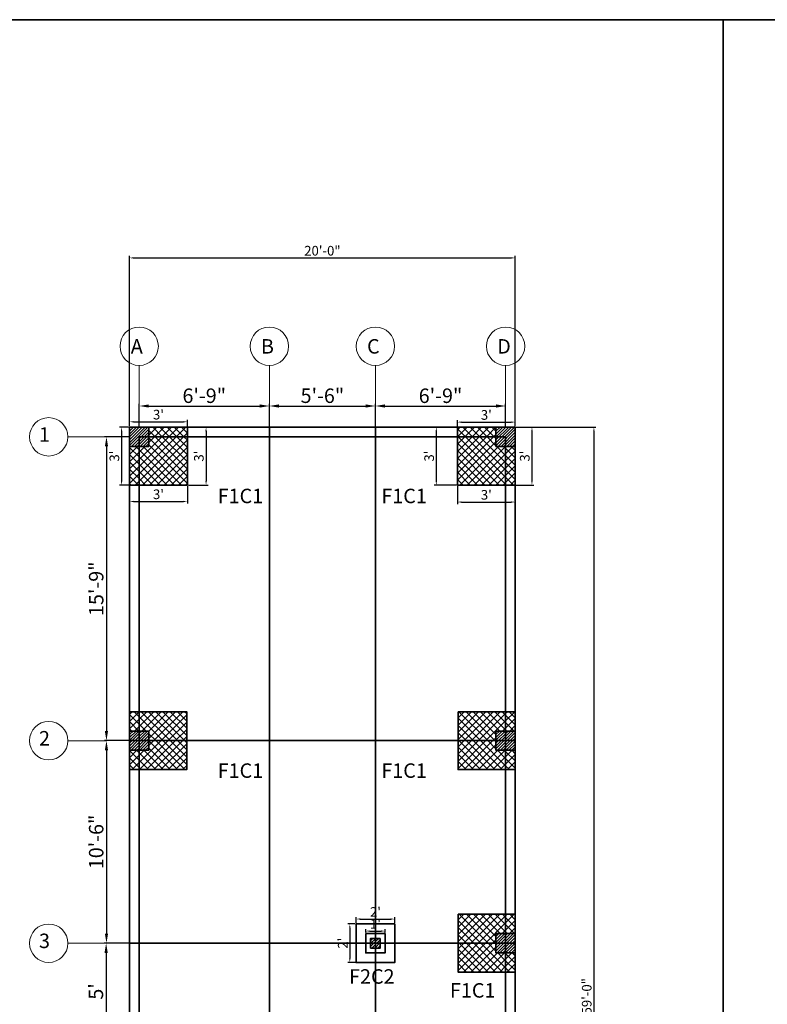
# Model space of a CAD drawing. Units: millimetres. Extents: x 20768 to 23556, y 50760 to 52704.
# Tile 35 of 36: x 22556 to 23021, y 52092 to 52704. Entities that reach past the tile are written whole.
import ezdxf

# ---------------------------------------------------------------- set-up
doc = ezdxf.new("R2010")
doc.units = ezdxf.units.MM
for name, color, linetype, lineweight in [('A-ANNO-TTLB', 7, 'Continuous', 35), ('S-ANNO-DIMS', 2, 'Continuous', 18), ('S-ANNO-TEXT', 6, 'Continuous', 18), ('S-BEAM', 3, 'Continuous', 35), ('S-COLS', 20, 'Continuous', 35), ('S-COLS-PATT', 8, 'Continuous', 13), ('S-FNDN', 200, 'Continuous', 35), ('S-GRID', 1, 'Continuous', 18)]:
    doc.layers.add(name, color=color, linetype=linetype, lineweight=lineweight)
doc.styles.get("Standard").update_dxf_attribs({"font": 'arial.ttf'})
doc.dimstyles.new('ISO-25', dxfattribs={"dimtxt": 6, "dimasz": 2.5, "dimexe": 1.25, "dimexo": 0.625, "dimtad": 1, "dimdec": 0, "dimlunit": 3, "dimtxsty": 'Standard', "dimcen": 2.5, "dimadec": 0, "dimazin": 0, "dimtfac": 1, "dimtdec": 0, "dimtmove": 0, "dimatfit": 3, "dimfxl": 1, "dimarcsym": 0})
pattern_1 = [(45, (568.6884, 0), (-0.898025612, 0.898025612), [])]
pattern_2 = [(45, (-102.8262, 0), (-2.24506403, 2.24506403), []), (135, (-102.8262, 0), (-2.24506403, -2.24506403), [])]
pattern_3 = [(45, (-102.8262, 0), (-0.898025612, 0.898025612), [])]

# ---------------------------------------------------------------- blocks, each defined once
blk = doc.blocks.new('*D51')
at = {"layer": 'Defpoints', "color": 0, "transparency": 16777216}
for p in [(22710.96, 52463.68), (22629.96, 52450.51), (22710.96, 52450.51)]:
    blk.add_point(p, dxfattribs=at)
at = {"layer": 'S-ANNO-DIMS', "color": 0, "lineweight": -2, "transparency": 16777216}
for p, q in [((22629.96, 52451.13), (22629.96, 52464.93)), ((22710.96, 52451.13), (22710.96, 52464.93)), ((22635.96, 52463.68), (22704.96, 52463.68))]:
    blk.add_line(p, q, dxfattribs=at)
at = {"layer": 'S-ANNO-DIMS', "color": 0, "transparency": 16777216}
for points in [[(22635.96, 52464.68), (22635.96, 52462.68), (22629.96, 52463.68)], [(22704.96, 52464.68), (22704.96, 52462.68), (22710.96, 52463.68)]]:
    blk.add_solid(points, dxfattribs=at)
at = {"layer": 'S-ANNO-DIMS', "color": 0, "transparency": 16777216, "insert": (22670.46, 52468.9), "char_height": 9, "attachment_point": 5}
blk.add_mtext('6\'-9"', dxfattribs=at)
blk = doc.blocks.new('*D52')
at = {"layer": 'Defpoints', "color": 0, "transparency": 16777216}
for p in [(22776.96, 52463.68), (22710.96, 52450.51), (22776.96, 52450.51)]:
    blk.add_point(p, dxfattribs=at)
at = {"layer": 'S-ANNO-DIMS', "color": 0, "lineweight": -2, "transparency": 16777216}
for p, q in [((22710.96, 52451.13), (22710.96, 52464.93)), ((22776.96, 52451.13), (22776.96, 52464.93)), ((22716.96, 52463.68), (22770.96, 52463.68))]:
    blk.add_line(p, q, dxfattribs=at)
at = {"layer": 'S-ANNO-DIMS', "color": 0, "transparency": 16777216}
for points in [[(22716.96, 52464.68), (22716.96, 52462.68), (22710.96, 52463.68)], [(22770.96, 52464.68), (22770.96, 52462.68), (22776.96, 52463.68)]]:
    blk.add_solid(points, dxfattribs=at)
at = {"layer": 'S-ANNO-DIMS', "color": 0, "transparency": 16777216, "insert": (22743.96, 52468.9), "char_height": 9, "attachment_point": 5}
blk.add_mtext('5\'-6"', dxfattribs=at)
blk = doc.blocks.new('*D53')
at = {"layer": 'Defpoints', "color": 0, "transparency": 16777216}
for p in [(22857.96, 52463.68), (22776.96, 52450.51), (22857.96, 52450.51)]:
    blk.add_point(p, dxfattribs=at)
at = {"layer": 'S-ANNO-DIMS', "color": 0, "lineweight": -2, "transparency": 16777216}
for p, q in [((22776.96, 52451.13), (22776.96, 52464.93)), ((22857.96, 52451.13), (22857.96, 52464.93)), ((22782.96, 52463.68), (22851.96, 52463.68))]:
    blk.add_line(p, q, dxfattribs=at)
at = {"layer": 'S-ANNO-DIMS', "color": 0, "transparency": 16777216}
for points in [[(22782.96, 52464.68), (22782.96, 52462.68), (22776.96, 52463.68)], [(22851.96, 52464.68), (22851.96, 52462.68), (22857.96, 52463.68)]]:
    blk.add_solid(points, dxfattribs=at)
at = {"layer": 'S-ANNO-DIMS', "color": 0, "transparency": 16777216, "insert": (22817.46, 52468.9), "char_height": 9, "attachment_point": 5}
blk.add_mtext('6\'-9"', dxfattribs=at)
blk = doc.blocks.new('*D54')
at = {"layer": 'Defpoints', "color": 0, "transparency": 16777216}
for p in [(22623.96, 52444.51), (22609.6, 52255.51), (22623.96, 52255.51)]:
    blk.add_point(p, dxfattribs=at)
at = {"layer": 'S-ANNO-DIMS', "color": 0, "lineweight": -2, "transparency": 16777216}
for p, q in [((22623.34, 52444.51), (22608.35, 52444.51)), ((22609.6, 52438.51), (22609.6, 52261.51)), ((22623.34, 52255.51), (22608.35, 52255.51))]:
    blk.add_line(p, q, dxfattribs=at)
at = {"layer": 'S-ANNO-DIMS', "color": 0, "transparency": 16777216}
for points in [[(22608.6, 52438.51), (22610.6, 52438.51), (22609.6, 52444.51)], [(22608.6, 52261.51), (22610.6, 52261.51), (22609.6, 52255.51)]]:
    blk.add_solid(points, dxfattribs=at)
at = {"layer": 'S-ANNO-DIMS', "color": 0, "transparency": 16777216, "insert": (22604.38, 52350.01), "char_height": 9, "attachment_point": 5, "rotation": 90}
blk.add_mtext('15\'-9"', dxfattribs=at)
blk = doc.blocks.new('*D55')
at = {"layer": 'Defpoints', "color": 0, "transparency": 16777216}
for p in [(22623.96, 52255.51), (22609.6, 52129.51), (22623.96, 52129.51)]:
    blk.add_point(p, dxfattribs=at)
at = {"layer": 'S-ANNO-DIMS', "color": 0, "lineweight": -2, "transparency": 16777216}
for p, q in [((22623.34, 52255.51), (22608.35, 52255.51)), ((22609.6, 52249.51), (22609.6, 52135.51)), ((22623.34, 52129.51), (22608.35, 52129.51))]:
    blk.add_line(p, q, dxfattribs=at)
at = {"layer": 'S-ANNO-DIMS', "color": 0, "transparency": 16777216}
for points in [[(22608.6, 52249.51), (22610.6, 52249.51), (22609.6, 52255.51)], [(22608.6, 52135.51), (22610.6, 52135.51), (22609.6, 52129.51)]]:
    blk.add_solid(points, dxfattribs=at)
at = {"layer": 'S-ANNO-DIMS', "color": 0, "transparency": 16777216, "insert": (22604.38, 52192.51), "char_height": 9, "attachment_point": 5, "rotation": 90}
blk.add_mtext('10\'-6"', dxfattribs=at)
blk = doc.blocks.new('*D56')
at = {"layer": 'Defpoints', "color": 0, "transparency": 16777216}
for p in [(22623.96, 52129.51), (22609.39, 52069.51), (22623.96, 52069.51)]:
    blk.add_point(p, dxfattribs=at)
at = {"layer": 'S-ANNO-DIMS', "color": 0, "lineweight": -2, "transparency": 16777216}
for p, q in [((22623.34, 52129.51), (22608.14, 52129.51)), ((22609.39, 52123.51), (22609.39, 52075.51)), ((22623.34, 52069.51), (22608.14, 52069.51))]:
    blk.add_line(p, q, dxfattribs=at)
at = {"layer": 'S-ANNO-DIMS', "color": 0, "transparency": 16777216}
for points in [[(22608.39, 52123.51), (22610.39, 52123.51), (22609.39, 52129.51)], [(22608.39, 52075.51), (22610.39, 52075.51), (22609.39, 52069.51)]]:
    blk.add_solid(points, dxfattribs=at)
at = {"layer": 'S-ANNO-DIMS', "color": 0, "transparency": 16777216, "insert": (22604.19, 52099.51), "char_height": 9, "attachment_point": 5, "rotation": 90}
blk.add_mtext("5'", dxfattribs=at)
blk = doc.blocks.new('*D59')
at = {"layer": 'Defpoints', "color": 0, "transparency": 16777216}
for p in [(22623.96, 52414.51), (22659.96, 52414.51), (22659.96, 52404.3)]:
    blk.add_point(p, dxfattribs=at)
at = {"layer": 'S-ANNO-DIMS', "color": 0, "lineweight": -2, "transparency": 16777216}
for p, q in [((22623.96, 52413.88), (22623.96, 52403.05)), ((22659.96, 52413.88), (22659.96, 52403.05)), ((22626.46, 52404.3), (22657.46, 52404.3))]:
    blk.add_line(p, q, dxfattribs=at)
at = {"layer": 'S-ANNO-DIMS', "color": 0, "transparency": 16777216}
for points in [[(22626.46, 52404.72), (22626.46, 52403.89), (22623.96, 52404.3)], [(22657.46, 52404.72), (22657.46, 52403.89), (22659.96, 52404.3)]]:
    blk.add_solid(points, dxfattribs=at)
at = {"layer": 'S-ANNO-DIMS', "color": 0, "transparency": 16777216, "insert": (22641.96, 52407.99), "char_height": 6, "attachment_point": 5}
blk.add_mtext("3'", dxfattribs=at)
blk = doc.blocks.new('*D60')
at = {"layer": 'Defpoints', "color": 0, "transparency": 16777216}
for p in [(22659.96, 52450.51), (22659.96, 52414.51), (22671.57, 52414.51)]:
    blk.add_point(p, dxfattribs=at)
at = {"layer": 'S-ANNO-DIMS', "color": 0, "lineweight": -2, "transparency": 16777216}
for p, q in [((22660.59, 52450.51), (22672.82, 52450.51)), ((22671.57, 52448.01), (22671.57, 52417.01)), ((22660.59, 52414.51), (22672.82, 52414.51))]:
    blk.add_line(p, q, dxfattribs=at)
at = {"layer": 'S-ANNO-DIMS', "color": 0, "transparency": 16777216}
for points in [[(22671.15, 52448.01), (22671.98, 52448.01), (22671.57, 52450.51)], [(22671.15, 52417.01), (22671.98, 52417.01), (22671.57, 52414.51)]]:
    blk.add_solid(points, dxfattribs=at)
at = {"layer": 'S-ANNO-DIMS', "color": 0, "transparency": 16777216, "insert": (22667.88, 52432.51), "char_height": 6, "attachment_point": 5, "rotation": 90}
blk.add_mtext("3'", dxfattribs=at)
blk = doc.blocks.new('*D61')
at = {"layer": 'Defpoints', "color": 0, "transparency": 16777216}
for p in [(22659.96, 52453.85), (22623.96, 52450.51), (22659.96, 52450.51)]:
    blk.add_point(p, dxfattribs=at)
at = {"layer": 'S-ANNO-DIMS', "color": 0, "lineweight": -2, "transparency": 16777216}
for p, q in [((22623.96, 52451.13), (22623.96, 52455.1)), ((22626.46, 52453.85), (22657.46, 52453.85)), ((22659.96, 52451.13), (22659.96, 52455.1))]:
    blk.add_line(p, q, dxfattribs=at)
at = {"layer": 'S-ANNO-DIMS', "color": 0, "transparency": 16777216}
for points in [[(22626.46, 52454.27), (22626.46, 52453.43), (22623.96, 52453.85)], [(22657.46, 52454.27), (22657.46, 52453.43), (22659.96, 52453.85)]]:
    blk.add_solid(points, dxfattribs=at)
at = {"layer": 'S-ANNO-DIMS', "color": 0, "transparency": 16777216, "insert": (22641.96, 52457.54), "char_height": 6, "attachment_point": 5}
blk.add_mtext("3'", dxfattribs=at)
blk = doc.blocks.new('*D48')
at = {"layer": 'Defpoints', "color": 0, "transparency": 16777216}
for p in [(22623.96, 52450.51), (22619.01, 52414.51), (22623.96, 52414.51)]:
    blk.add_point(p, dxfattribs=at)
at = {"layer": 'S-ANNO-DIMS', "color": 0, "lineweight": -2, "transparency": 16777216}
for p, q in [((22623.34, 52450.51), (22617.76, 52450.51)), ((22619.01, 52448.01), (22619.01, 52417.01)), ((22623.34, 52414.51), (22617.76, 52414.51))]:
    blk.add_line(p, q, dxfattribs=at)
at = {"layer": 'S-ANNO-DIMS', "color": 0, "transparency": 16777216}
for points in [[(22618.59, 52448.01), (22619.42, 52448.01), (22619.01, 52450.51)], [(22618.59, 52417.01), (22619.42, 52417.01), (22619.01, 52414.51)]]:
    blk.add_solid(points, dxfattribs=at)
at = {"layer": 'S-ANNO-DIMS', "color": 0, "transparency": 16777216, "insert": (22615.31, 52432.51), "char_height": 6, "attachment_point": 5, "rotation": 90}
blk.add_mtext("3'", dxfattribs=at)
blk = doc.blocks.new('*D62')
at = {"layer": 'Defpoints', "color": 0, "transparency": 16777216}
for p in [(22827.96, 52450.51), (22814.83, 52414.51), (22827.96, 52414.51)]:
    blk.add_point(p, dxfattribs=at)
at = {"layer": 'S-ANNO-DIMS', "color": 0, "lineweight": -2, "transparency": 16777216}
for p, q in [((22827.34, 52450.51), (22813.58, 52450.51)), ((22814.83, 52448.01), (22814.83, 52417.01)), ((22827.34, 52414.51), (22813.58, 52414.51))]:
    blk.add_line(p, q, dxfattribs=at)
at = {"layer": 'S-ANNO-DIMS', "color": 0, "transparency": 16777216}
for points in [[(22814.41, 52448.01), (22815.25, 52448.01), (22814.83, 52450.51)], [(22814.41, 52417.01), (22815.25, 52417.01), (22814.83, 52414.51)]]:
    blk.add_solid(points, dxfattribs=at)
at = {"layer": 'S-ANNO-DIMS', "color": 0, "transparency": 16777216, "insert": (22811.14, 52432.51), "char_height": 6, "attachment_point": 5, "rotation": 90}
blk.add_mtext("3'", dxfattribs=at)
blk = doc.blocks.new('*D63')
at = {"layer": 'Defpoints', "color": 0, "transparency": 16777216}
for p in [(22827.96, 52414.51), (22863.96, 52414.51), (22863.96, 52403.95)]:
    blk.add_point(p, dxfattribs=at)
at = {"layer": 'S-ANNO-DIMS', "color": 0, "lineweight": -2, "transparency": 16777216}
for p, q in [((22827.96, 52413.88), (22827.96, 52402.7)), ((22863.96, 52413.88), (22863.96, 52402.7)), ((22830.46, 52403.95), (22861.46, 52403.95))]:
    blk.add_line(p, q, dxfattribs=at)
at = {"layer": 'S-ANNO-DIMS', "color": 0, "transparency": 16777216}
for points in [[(22830.46, 52404.37), (22830.46, 52403.54), (22827.96, 52403.95)], [(22861.46, 52404.37), (22861.46, 52403.54), (22863.96, 52403.95)]]:
    blk.add_solid(points, dxfattribs=at)
at = {"layer": 'S-ANNO-DIMS', "color": 0, "transparency": 16777216, "insert": (22845.96, 52407.64), "char_height": 6, "attachment_point": 5}
blk.add_mtext("3'", dxfattribs=at)
blk = doc.blocks.new('*D64')
at = {"layer": 'Defpoints', "color": 0, "transparency": 16777216}
for p in [(22863.96, 52450.51), (22863.96, 52414.51), (22874.35, 52414.51)]:
    blk.add_point(p, dxfattribs=at)
at = {"layer": 'S-ANNO-DIMS', "color": 0, "lineweight": -2, "transparency": 16777216}
for p, q in [((22864.59, 52450.51), (22875.6, 52450.51)), ((22874.35, 52448.01), (22874.35, 52417.01)), ((22864.59, 52414.51), (22875.6, 52414.51))]:
    blk.add_line(p, q, dxfattribs=at)
at = {"layer": 'S-ANNO-DIMS', "color": 0, "transparency": 16777216}
for points in [[(22873.93, 52448.01), (22874.77, 52448.01), (22874.35, 52450.51)], [(22873.93, 52417.01), (22874.77, 52417.01), (22874.35, 52414.51)]]:
    blk.add_solid(points, dxfattribs=at)
at = {"layer": 'S-ANNO-DIMS', "color": 0, "transparency": 16777216, "insert": (22870.66, 52432.51), "char_height": 6, "attachment_point": 5, "rotation": 90}
blk.add_mtext("3'", dxfattribs=at)
blk = doc.blocks.new('*D49')
at = {"layer": 'Defpoints', "color": 0, "transparency": 16777216}
for p in [(22863.96, 52453.66), (22827.96, 52450.51), (22863.96, 52450.51)]:
    blk.add_point(p, dxfattribs=at)
at = {"layer": 'S-ANNO-DIMS', "color": 0, "lineweight": -2, "transparency": 16777216}
for p, q in [((22827.96, 52451.13), (22827.96, 52454.91)), ((22830.46, 52453.66), (22861.46, 52453.66)), ((22863.96, 52451.13), (22863.96, 52454.91))]:
    blk.add_line(p, q, dxfattribs=at)
at = {"layer": 'S-ANNO-DIMS', "color": 0, "transparency": 16777216}
for points in [[(22830.46, 52454.08), (22830.46, 52453.24), (22827.96, 52453.66)], [(22861.46, 52454.08), (22861.46, 52453.24), (22863.96, 52453.66)]]:
    blk.add_solid(points, dxfattribs=at)
at = {"layer": 'S-ANNO-DIMS', "color": 0, "transparency": 16777216, "insert": (22845.96, 52457.35), "char_height": 6, "attachment_point": 5}
blk.add_mtext("3'", dxfattribs=at)
blk = doc.blocks.new('*D65')
at = {"layer": 'Defpoints', "color": 0, "transparency": 16777216}
for p in [(22770.96, 52135.51), (22782.96, 52137.07), (22782.96, 52135.51)]:
    blk.add_point(p, dxfattribs=at)
at = {"layer": 'S-ANNO-DIMS', "color": 0, "lineweight": -2, "transparency": 16777216}
for p, q in [((22770.96, 52136.13), (22770.96, 52138.32)), ((22773.46, 52137.07), (22780.46, 52137.07)), ((22782.96, 52136.13), (22782.96, 52138.32))]:
    blk.add_line(p, q, dxfattribs=at)
at = {"layer": 'S-ANNO-DIMS', "color": 0, "transparency": 16777216}
for points in [[(22773.46, 52137.48), (22773.46, 52136.65), (22770.96, 52137.07)], [(22780.46, 52137.48), (22780.46, 52136.65), (22782.96, 52137.07)]]:
    blk.add_solid(points, dxfattribs=at)
at = {"layer": 'S-ANNO-DIMS', "color": 0, "transparency": 16777216, "insert": (22776.96, 52140.7), "char_height": 6, "attachment_point": 5}
blk.add_mtext("1'", dxfattribs=at)
blk = doc.blocks.new('*D66')
at = {"layer": 'Defpoints', "color": 0, "transparency": 16777216}
for p in [(22764.96, 52141.51), (22788.96, 52144.54), (22788.96, 52141.51)]:
    blk.add_point(p, dxfattribs=at)
at = {"layer": 'S-ANNO-DIMS', "color": 0, "lineweight": -2, "transparency": 16777216}
for p, q in [((22764.96, 52142.13), (22764.96, 52145.79)), ((22767.46, 52144.54), (22786.46, 52144.54)), ((22788.96, 52142.13), (22788.96, 52145.79))]:
    blk.add_line(p, q, dxfattribs=at)
at = {"layer": 'S-ANNO-DIMS', "color": 0, "transparency": 16777216}
for points in [[(22767.46, 52144.95), (22767.46, 52144.12), (22764.96, 52144.54)], [(22786.46, 52144.95), (22786.46, 52144.12), (22788.96, 52144.54)]]:
    blk.add_solid(points, dxfattribs=at)
at = {"layer": 'S-ANNO-DIMS', "color": 0, "transparency": 16777216, "insert": (22776.96, 52148.17), "char_height": 6, "attachment_point": 5}
blk.add_mtext("2'", dxfattribs=at)
blk = doc.blocks.new('*D67')
at = {"layer": 'Defpoints', "color": 0, "transparency": 16777216}
for p in [(22764.96, 52141.51), (22761.03, 52117.51), (22764.96, 52117.51)]:
    blk.add_point(p, dxfattribs=at)
at = {"layer": 'S-ANNO-DIMS', "color": 0, "lineweight": -2, "transparency": 16777216}
for p, q in [((22764.34, 52141.51), (22759.78, 52141.51)), ((22761.03, 52139.01), (22761.03, 52120.01)), ((22764.34, 52117.51), (22759.78, 52117.51))]:
    blk.add_line(p, q, dxfattribs=at)
at = {"layer": 'S-ANNO-DIMS', "color": 0, "transparency": 16777216}
for points in [[(22760.61, 52139.01), (22761.44, 52139.01), (22761.03, 52141.51)], [(22760.61, 52120.01), (22761.44, 52120.01), (22761.03, 52117.51)]]:
    blk.add_solid(points, dxfattribs=at)
at = {"layer": 'S-ANNO-DIMS', "color": 0, "transparency": 16777216, "insert": (22757.39, 52129.51), "char_height": 6, "attachment_point": 5, "rotation": 90}
blk.add_mtext("2'", dxfattribs=at)
blk = doc.blocks.new('GRID-BUBBLE')
blk.add_line((47.87, 11.93), (23.87, 11.93))
blk.add_circle((11.93, 11.93), 11.93)
blk = doc.blocks.new('*D225')
at = {"layer": 'Defpoints', "color": 0, "transparency": 16777216}
for p in [(22863.96, 52555.8), (22623.96, 52450.51), (22863.96, 52450.51)]:
    blk.add_point(p, dxfattribs=at)
at = {"layer": 'S-ANNO-DIMS', "color": 0, "lineweight": -2, "transparency": 16777216}
for p, q in [((22623.96, 52451.13), (22623.96, 52557.05)), ((22863.96, 52451.13), (22863.96, 52557.05)), ((22626.46, 52555.8), (22861.46, 52555.8))]:
    blk.add_line(p, q, dxfattribs=at)
at = {"layer": 'S-ANNO-DIMS', "color": 0, "transparency": 16777216}
for points in [[(22626.46, 52556.22), (22626.46, 52555.38), (22623.96, 52555.8)], [(22861.46, 52556.22), (22861.46, 52555.38), (22863.96, 52555.8)]]:
    blk.add_solid(points, dxfattribs=at)
at = {"layer": 'S-ANNO-DIMS', "color": 0, "transparency": 16777216, "insert": (22743.96, 52559.49), "char_height": 6, "attachment_point": 5}
blk.add_mtext('20\'-0"', dxfattribs=at)
blk = doc.blocks.new('*D226')
at = {"layer": 'Defpoints', "color": 0, "transparency": 16777216}
for p in [(22863.96, 52450.51), (22863.96, 51742.51), (22912.89, 51742.51)]:
    blk.add_point(p, dxfattribs=at)
at = {"layer": 'S-ANNO-DIMS', "color": 0, "lineweight": -2, "transparency": 16777216}
for p, q in [((22864.59, 52450.51), (22914.14, 52450.51)), ((22912.89, 52448.01), (22912.89, 51745.01)), ((22864.59, 51742.51), (22914.14, 51742.51))]:
    blk.add_line(p, q, dxfattribs=at)
at = {"layer": 'S-ANNO-DIMS', "color": 0, "transparency": 16777216}
for points in [[(22912.48, 52448.01), (22913.31, 52448.01), (22912.89, 52450.51)], [(22912.48, 51745.01), (22913.31, 51745.01), (22912.89, 51742.51)]]:
    blk.add_solid(points, dxfattribs=at)
at = {"layer": 'S-ANNO-DIMS', "color": 0, "transparency": 16777216, "insert": (22909.21, 52096.51), "char_height": 6, "attachment_point": 5, "rotation": 90}
blk.add_mtext('59\'-0"', dxfattribs=at)

msp = doc.modelspace()

# ---------------------------------------------------------------- hatches: boundary and pattern name
at = {"layer": 'S-COLS-PATT'}
h = msp.add_hatch(dxfattribs=at)
h.set_pattern_fill('ANSI31', color=256, scale=0.4)
h.set_pattern_definition(pattern_1)
h.paths.add_polyline_path([(22635.96, 52450.51), (22623.96, 52450.51), (22623.96, 52438.51), (22629.96, 52438.51), (22629.96, 52444.51), (22635.96, 52444.51)])
h = msp.add_hatch(dxfattribs=at)
h.set_pattern_fill('ANSI37', color=256)
h.set_pattern_definition(pattern_2)
h.paths.add_polyline_path([(22659.96, 52450.51), (22635.96, 52450.51), (22635.96, 52444.51), (22659.96, 52444.51)])
h = msp.add_hatch(dxfattribs=at)
h.set_pattern_fill('ANSI37', color=256)
h.set_pattern_definition(pattern_2)
h.paths.add_polyline_path([(22851.96, 52450.51), (22827.96, 52450.51), (22827.96, 52444.51), (22851.96, 52444.51)])
h = msp.add_hatch(dxfattribs=at)
h.set_pattern_fill('ANSI31', color=256, scale=0.4)
h.set_pattern_definition(pattern_1)
h.paths.add_polyline_path([(22863.96, 52450.51), (22851.96, 52450.51), (22851.96, 52438.51), (22863.96, 52438.51)])
h = msp.add_hatch(dxfattribs=at)
h.set_pattern_fill('ANSI31', color=256, scale=0.4)
h.set_pattern_definition(pattern_1)
h.paths.add_polyline_path([(22635.96, 52444.51), (22629.96, 52444.51), (22629.96, 52438.51), (22635.96, 52438.51)], flags=17)
h = msp.add_hatch(dxfattribs=at)
h.set_pattern_fill('ANSI37', color=256)
h.set_pattern_definition(pattern_2)
h.paths.add_polyline_path([(22659.96, 52444.51), (22635.96, 52444.51), (22635.96, 52438.51), (22629.96, 52438.51), (22629.96, 52414.51), (22659.96, 52414.51)])
h = msp.add_hatch(dxfattribs=at)
h.set_pattern_fill('ANSI37', color=256)
h.set_pattern_definition(pattern_2)
h.paths.add_polyline_path([(22857.96, 52438.51), (22851.96, 52438.51), (22851.96, 52444.51), (22827.96, 52444.51), (22827.96, 52414.51), (22857.96, 52414.51)])
h = msp.add_hatch(dxfattribs=at)
h.set_pattern_fill('ANSI37', color=256)
h.set_pattern_definition(pattern_2)
h.paths.add_polyline_path([(22629.96, 52438.51), (22623.96, 52438.51), (22623.96, 52414.51), (22629.96, 52414.51)])
h = msp.add_hatch(dxfattribs=at)
h.set_pattern_fill('ANSI37', color=256)
h.set_pattern_definition(pattern_2)
h.paths.add_polyline_path([(22863.96, 52438.51), (22857.96, 52438.51), (22857.96, 52414.51), (22863.96, 52414.51)])
h = msp.add_hatch(dxfattribs=at)
h.set_pattern_fill('ANSI37', color=256)
h.set_pattern_definition(pattern_2)
h.paths.add_polyline_path([(22629.96, 52273.51), (22623.96, 52273.51), (22623.96, 52261.51), (22629.96, 52261.51)])
h = msp.add_hatch(dxfattribs=at)
h.set_pattern_fill('ANSI37', color=256)
h.set_pattern_definition(pattern_2)
h.paths.add_polyline_path([(22659.53, 52273.51), (22629.96, 52273.51), (22629.96, 52261.51), (22635.96, 52261.51), (22635.96, 52255.51), (22659.53, 52255.51)])
h = msp.add_hatch(dxfattribs=at)
h.set_pattern_fill('ANSI37', color=256)
h.set_pattern_definition(pattern_2)
h.paths.add_polyline_path([(22857.96, 52273.51), (22828.39, 52273.51), (22828.39, 52255.51), (22851.96, 52255.51), (22851.96, 52261.51), (22857.96, 52261.51)])
h = msp.add_hatch(dxfattribs=at)
h.set_pattern_fill('ANSI37', color=256)
h.set_pattern_definition(pattern_2)
h.paths.add_polyline_path([(22863.96, 52273.51), (22857.96, 52273.51), (22857.96, 52261.51), (22863.96, 52261.51)])
h = msp.add_hatch(dxfattribs=at)
h.set_pattern_fill('ANSI31', color=256, scale=0.4)
h.set_pattern_definition(pattern_3)
h.paths.add_polyline_path([(22629.96, 52261.51), (22623.96, 52261.51), (22623.96, 52255.51), (22629.96, 52255.51)])
h = msp.add_hatch(dxfattribs=at)
h.set_pattern_fill('ANSI31', color=256, scale=0.4)
h.set_pattern_definition(pattern_3)
h.paths.add_polyline_path([(22635.96, 52261.51), (22629.96, 52261.51), (22629.96, 52255.51), (22635.96, 52255.51)])
h = msp.add_hatch(dxfattribs=at)
h.set_pattern_fill('ANSI31', color=256, scale=0.4)
h.set_pattern_definition(pattern_1)
h.paths.add_polyline_path([(22863.96, 52261.51), (22851.96, 52261.51), (22851.96, 52249.51), (22863.96, 52249.51)])
h = msp.add_hatch(dxfattribs=at)
h.set_pattern_fill('ANSI31', color=256, scale=0.4)
h.set_pattern_definition(pattern_3)
h.paths.add_polyline_path([(22629.96, 52255.51), (22623.96, 52255.51), (22623.96, 52249.51), (22629.96, 52249.51)])
h = msp.add_hatch(dxfattribs=at)
h.set_pattern_fill('ANSI37', color=256)
h.set_pattern_definition(pattern_2)
h.paths.add_polyline_path([(22659.53, 52255.51), (22635.96, 52255.51), (22635.96, 52249.51), (22629.96, 52249.51), (22629.96, 52237.51), (22659.53, 52237.51)])
h = msp.add_hatch(dxfattribs=at)
h.set_pattern_fill('ANSI31', color=256, scale=0.4)
h.set_pattern_definition(pattern_3)
h.paths.add_polyline_path([(22635.96, 52255.51), (22629.96, 52255.51), (22629.96, 52249.51), (22635.96, 52249.51)])
h = msp.add_hatch(dxfattribs=at)
h.set_pattern_fill('ANSI37', color=256)
h.set_pattern_definition(pattern_2)
h.paths.add_polyline_path([(22851.96, 52255.51), (22828.39, 52255.51), (22828.39, 52237.51), (22857.96, 52237.51), (22857.96, 52249.51), (22851.96, 52249.51)])
h = msp.add_hatch(dxfattribs=at)
h.set_pattern_fill('ANSI37', color=256)
h.set_pattern_definition(pattern_2)
h.paths.add_polyline_path([(22629.96, 52249.51), (22623.96, 52249.51), (22623.96, 52237.51), (22629.96, 52237.51)])
h = msp.add_hatch(dxfattribs=at)
h.set_pattern_fill('ANSI37', color=256)
h.set_pattern_definition(pattern_2)
h.paths.add_polyline_path([(22863.96, 52249.51), (22857.96, 52249.51), (22857.96, 52237.51), (22863.96, 52237.51)])
h = msp.add_hatch(dxfattribs=at)
h.set_pattern_fill('ANSI37', color=256)
h.set_pattern_definition(pattern_2)
h.paths.add_polyline_path([(22851.96, 52135.51), (22857.96, 52135.51), (22857.96, 52147.51), (22828.39, 52147.51), (22828.39, 52129.51), (22851.96, 52129.51)])
h = msp.add_hatch(dxfattribs=at)
h.set_pattern_fill('ANSI37', color=256)
h.set_pattern_definition(pattern_2)
h.paths.add_polyline_path([(22863.96, 52147.51), (22857.96, 52147.51), (22857.96, 52135.51), (22863.96, 52135.51)])
h = msp.add_hatch(dxfattribs=at)
h.set_pattern_fill('ANSI31', color=256, scale=0.4)
h.set_pattern_definition(pattern_1)
h.paths.add_polyline_path([(22863.96, 52135.51), (22851.96, 52135.51), (22851.96, 52123.51), (22863.96, 52123.51)])
h = msp.add_hatch(dxfattribs=at)
h.set_pattern_fill('ANSI31', color=256, scale=0.4)
h.set_pattern_definition(pattern_1)
h.paths.add_polyline_path([(22776.96, 52132.51), (22773.96, 52132.51), (22773.96, 52129.51), (22776.96, 52129.51)])
h = msp.add_hatch(dxfattribs=at)
h.set_pattern_fill('ANSI31', color=256, scale=0.4)
h.set_pattern_definition(pattern_1)
h.paths.add_polyline_path([(22776.96, 52129.51), (22773.96, 52129.51), (22773.96, 52126.51), (22776.96, 52126.51)], flags=17)
h = msp.add_hatch(dxfattribs=at)
h.set_pattern_fill('ANSI31', color=256, scale=0.4)
h.set_pattern_definition(pattern_1)
h.paths.add_polyline_path([(22779.96, 52132.51), (22776.96, 52132.51), (22776.96, 52129.51), (22779.96, 52129.51)])
h = msp.add_hatch(dxfattribs=at)
h.set_pattern_fill('ANSI31', color=256, scale=0.4)
h.set_pattern_definition(pattern_1)
h.paths.add_polyline_path([(22779.96, 52129.51), (22776.96, 52129.51), (22776.96, 52126.51), (22779.96, 52126.51)])
h = msp.add_hatch(dxfattribs=at)
h.set_pattern_fill('ANSI37', color=256)
h.set_pattern_definition(pattern_2)
h.paths.add_polyline_path([(22857.96, 52123.51), (22851.96, 52123.51), (22851.96, 52129.51), (22828.39, 52129.51), (22828.39, 52111.51), (22857.96, 52111.51)])
h = msp.add_hatch(dxfattribs=at)
h.set_pattern_fill('ANSI37', color=256)
h.set_pattern_definition(pattern_2)
h.paths.add_polyline_path([(22863.96, 52123.51), (22857.96, 52123.51), (22857.96, 52111.51), (22863.96, 52111.51)])

# ---------------------------------------------------------------- linework, layer by layer
at = {"layer": 'A-ANNO-TTLB'}
msp.add_line((22993.36, 52703.98), (22993.36, 51623.53), dxfattribs=at)
msp.add_lwpolyline([(20768.14, 52703.98), (23555.8, 52703.98), (23555.8, 51623.53), (20768.14, 51623.53)], close=True, dxfattribs=at)
at = {"layer": 'S-BEAM'}
for p, q in [((22710.96, 52450.51), (22710.96, 51748.51)), ((22776.96, 52450.51), (22776.96, 51748.51)), ((22629.96, 52444.51), (22629.96, 51742.51)), ((22629.96, 52444.51), (22857.96, 52444.51)), ((22857.96, 52444.51), (22857.96, 52261.51)), ((22857.96, 52261.51), (22857.96, 52135.51)), ((22623.96, 52255.51), (22863.96, 52255.51)), ((22857.96, 52135.51), (22857.96, 51823.51)), ((22623.96, 52129.51), (22863.96, 52129.51))]:
    msp.add_line(p, q, dxfattribs=at)
at = {"layer": 'S-COLS'}
for points in [[(22623.96, 52450.51), (22635.96, 52450.51), (22635.96, 52438.51), (22623.96, 52438.51)], [(22623.96, 52450.51), (22659.96, 52450.51), (22659.96, 52414.51), (22623.96, 52414.51)], [(22827.96, 52450.51), (22863.96, 52450.51), (22863.96, 52414.51), (22827.96, 52414.51)], [(22851.96, 52450.51), (22863.96, 52450.51), (22863.96, 52438.51), (22851.96, 52438.51)], [(22623.96, 52273.51), (22659.53, 52273.51), (22659.53, 52237.51), (22623.96, 52237.51)], [(22828.39, 52273.51), (22863.96, 52273.51), (22863.96, 52237.51), (22828.39, 52237.51)], [(22635.96, 52261.51), (22623.96, 52261.51), (22623.96, 52249.51), (22635.96, 52249.51)], [(22851.96, 52261.51), (22863.96, 52261.51), (22863.96, 52249.51), (22851.96, 52249.51)], [(22828.39, 52147.51), (22863.96, 52147.51), (22863.96, 52111.51), (22828.39, 52111.51)], [(22764.96, 52141.51), (22788.96, 52141.51), (22788.96, 52117.51), (22764.96, 52117.51)], [(22770.96, 52135.51), (22782.96, 52135.51), (22782.96, 52123.51), (22770.96, 52123.51)], [(22851.96, 52135.51), (22863.96, 52135.51), (22863.96, 52123.51), (22851.96, 52123.51)], [(22779.96, 52132.51), (22773.96, 52132.51), (22773.96, 52126.51), (22779.96, 52126.51)]]:
    msp.add_lwpolyline(points, close=True, dxfattribs=at)
at = {"layer": 'S-FNDN'}
for p, q in [((22623.96, 52450.51), (22863.96, 52450.51)), ((22623.96, 52450.51), (22623.96, 51742.51)), ((22863.96, 52450.51), (22863.96, 51742.51))]:
    msp.add_line(p, q, dxfattribs=at)
at = {"layer": 'S-GRID'}
for p, q in [((22629.96, 52464.93), (22629.96, 52488.93)), ((22710.96, 52464.93), (22710.96, 52488.93)), ((22776.96, 52464.93), (22776.96, 52488.93)), ((22857.96, 52464.93), (22857.96, 52488.93))]:
    msp.add_line(p, q, dxfattribs=at)
for centre in [(22629.96, 52500.87), (22710.96, 52500.87), (22776.96, 52500.87), (22857.96, 52500.87)]:
    msp.add_circle(centre, 11.93, dxfattribs=at)

# ---------------------------------------------------------------- block references
for p in [(22561.73, 52432.57), (22561.73, 52243.57), (22561.73, 52117.57)]:
    msp.add_blockref('GRID-BUBBLE', p, dxfattribs=at)

# ---------------------------------------------------------------- texts
at = {"layer": 'S-ANNO-TEXT', "char_height": 9, "attachment_point": 1}
for s, width, insert in [('  A', 27.5349, (22619.24, 52505.28)), ('  B', 27.5349, (22700.24, 52505.28)), ('  C', 27.5349, (22766.24, 52505.28)), ('  D', 27.5349, (22847.24, 52505.28)), ('  1', 27.5349, (22562.12, 52450.48)), ('F1C1', 26.4582, (22678.84, 52412.22)), ('F1C1', 26.4582, (22780.67, 52412.22)), ('  2', 27.5349, (22562.12, 52261.48)), ('F1C1', 26.4582, (22678.84, 52241.38)), ('F1C1', 26.4582, (22780.67, 52241.38)), ('  3', 27.5349, (22562.12, 52135.48)), ('F2C2', 26.4582, (22760.61, 52113.32)), ('F1C1', 26.4582, (22823.37, 52104.66))]:
    msp.add_mtext_dynamic_manual_height_columns(s, width=width, gutter_width=12.5, heights=[0], dxfattribs=dict(at, insert=insert))

# ---------------------------------------------------------------- dimensions: what is measured, and where the dimension line sits
at = {"layer": 'S-ANNO-DIMS'}
for base, p1, p2, override, picture, middle in [((22863.96, 52555.8), (22623.96, 52450.51), (22863.96, 52450.51), {"dimdec": 1, "dimlfac": 1, "dimrnd": 0, "dimzin": 1, "dimdsep": 46, "dimlunit": 4, "dimfrac": 2}, '*D225', (22743.96, 52559.49)), ((22710.96, 52463.68), (22629.96, 52450.51), (22710.96, 52450.51), {"dimtxt": 9, "dimasz": 6, "dimclrd": 0, "dimclre": 0, "dimclrt": 0}, '*D51', (22670.46, 52468.9)), ((22776.96, 52463.68), (22710.96, 52450.51), (22776.96, 52450.51), {"dimtxt": 9, "dimasz": 6, "dimclrd": 0, "dimclre": 0, "dimclrt": 0}, '*D52', (22743.96, 52468.9)), ((22857.96, 52463.68), (22776.96, 52450.51), (22857.96, 52450.51), {"dimtxt": 9, "dimasz": 6, "dimclrd": 0, "dimclre": 0, "dimclrt": 0}, '*D53', (22817.46, 52468.9)), ((22659.96, 52453.85), (22623.96, 52450.51), (22659.96, 52450.51), {"dimclrd": 0, "dimclre": 0, "dimclrt": 0}, '*D61', (22641.96, 52457.54)), ((22863.96, 52453.66), (22827.96, 52450.51), (22863.96, 52450.51), {"dimclrd": 0, "dimclre": 0, "dimclrt": 0}, '*D49', (22845.96, 52457.35)), ((22659.96, 52404.3), (22623.96, 52414.51), (22659.96, 52414.51), {"dimclrd": 0, "dimclre": 0, "dimclrt": 0}, '*D59', (22641.96, 52407.99)), ((22863.96, 52403.95), (22827.96, 52414.51), (22863.96, 52414.51), {"dimclrd": 0, "dimclre": 0, "dimclrt": 0}, '*D63', (22845.96, 52407.64)), ((22788.96, 52144.54), (22764.96, 52141.51), (22788.96, 52141.51), {"dimclrd": 0, "dimclre": 0, "dimclrt": 0}, '*D66', (22776.96, 52148.17)), ((22782.96, 52137.07), (22770.96, 52135.51), (22782.96, 52135.51), {"dimclrd": 0, "dimclre": 0, "dimclrt": 0}, '*D65', (22776.96, 52140.7))]:
    dim = msp.add_linear_dim(base=base, p1=p1, p2=p2, dimstyle='ISO-25', override=override, dxfattribs=at)
    dim.commit()
    dim.dimension.update_dxf_attribs({"geometry": picture, "text_midpoint": middle})
for base, p1, p2, override, picture, middle in [((22619.01, 52414.51), (22623.96, 52450.51), (22623.96, 52414.51), {"dimclrd": 0, "dimclre": 0, "dimclrt": 0}, '*D48', (22615.31, 52432.51)), ((22671.57, 52414.51), (22659.96, 52450.51), (22659.96, 52414.51), {"dimclrd": 0, "dimclre": 0, "dimclrt": 0}, '*D60', (22667.88, 52432.51)), ((22814.83, 52414.51), (22827.96, 52450.51), (22827.96, 52414.51), {"dimclrd": 0, "dimclre": 0, "dimclrt": 0}, '*D62', (22811.14, 52432.51)), ((22874.35, 52414.51), (22863.96, 52450.51), (22863.96, 52414.51), {"dimclrd": 0, "dimclre": 0, "dimclrt": 0}, '*D64', (22870.66, 52432.51)), ((22912.89, 51742.51), (22863.96, 52450.51), (22863.96, 51742.51), {"dimdec": 1, "dimlfac": 1, "dimrnd": 0, "dimzin": 1, "dimdsep": 46, "dimlunit": 4, "dimfrac": 2}, '*D226', (22909.21, 52096.51)), ((22609.6, 52255.51), (22623.96, 52444.51), (22623.96, 52255.51), {"dimtxt": 9, "dimasz": 6, "dimclrd": 0, "dimclre": 0, "dimclrt": 0}, '*D54', (22604.38, 52350.01)), ((22609.6, 52129.51), (22623.96, 52255.51), (22623.96, 52129.51), {"dimtxt": 9, "dimasz": 6, "dimclrd": 0, "dimclre": 0, "dimclrt": 0}, '*D55', (22604.38, 52192.51)), ((22761.03, 52117.51), (22764.96, 52141.51), (22764.96, 52117.51), {"dimclrd": 0, "dimclre": 0, "dimclrt": 0}, '*D67', (22757.39, 52129.51)), ((22609.39, 52069.51), (22623.96, 52129.51), (22623.96, 52069.51), {"dimtxt": 9, "dimasz": 6, "dimclrd": 0, "dimclre": 0, "dimclrt": 0}, '*D56', (22604.19, 52099.51))]:
    dim = msp.add_linear_dim(base=base, p1=p1, p2=p2, angle=90, dimstyle='ISO-25', override=override, dxfattribs=at)
    dim.commit()
    dim.dimension.update_dxf_attribs({"geometry": picture, "text_midpoint": middle})

doc.saveas('drawing.dxf')
